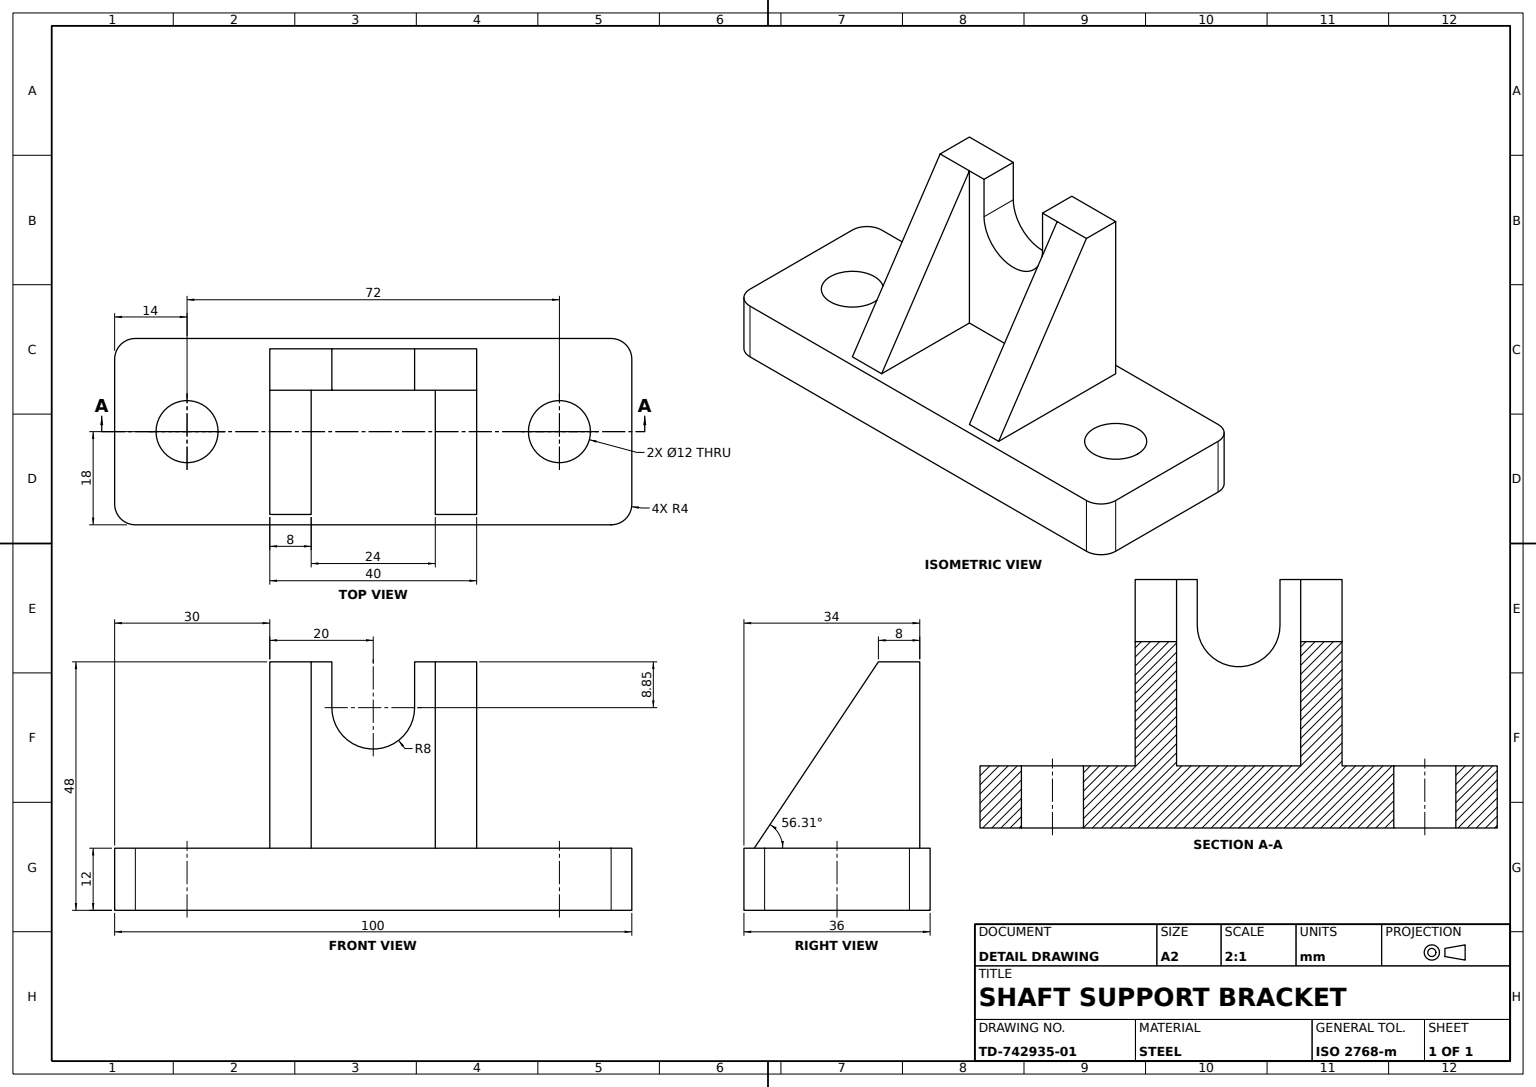
SolidWorks part; units mm, degrees
material "Plain Carbon Steel"
ref_plane "Front Plane" through (0, 0, 0) normal (0, 0, 1) x (1, 0, 0)
ref_plane "Top Plane" through (0, 0, 0) normal (0, 1, 0) x (1, 0, 0)
ref_plane "Right Plane" through (0, 0, 0) normal (1, 0, 0) x (0, 0, -1)
sketch "Base Plate Profile" plane through (0, 0, 0) normal (0, 0, 1) x (1, 0, 0)
  line L0 (0, 0) -> (50, 0)
  line L1 (50, 0) -> (50, 12)
  line L2 (50, 12) -> (-50, 12)
  line L3 (-50, 12) -> (-50, 0)
  line L4 (-50, 0) -> (0, 0)
  dimension "D1" = 100
  dimension "D2" = 12
  dimension "D3" = 50
extrude "Base Plate" add sketch "Base Plate Profile" along normal mid plane 36
sketch "Base Corners and Holes Sketch" plane through (0, 12, 0) normal (0, 1, 0) x (1, 0, 0)
  line L2 (-50, -14) -> (-50, -18)
  line L4 (-50, -18) -> (-46, -18)
  line L5 (50, 18) -> (-50, 18) construction
  line L6 (0, 18) -> (0, 0) construction
  line L7 (0, 0) -> (-26.4837, 0) construction
  line L8 (50, -14) -> (50, -18)
  line L9 (50, -18) -> (46, -18)
  line L10 (50, 14) -> (50, 18)
  line L11 (50, 18) -> (46, 18)
  line L12 (-50, 18) -> (-46, 18)
  line L13 (-50, 14) -> (-50, 18)
  arc A0 (-50, -14) -> (-46, -18) centre (-46, -14) ccw
  arc A1 (50, -14) -> (46, -18) centre (46, -14) cw
  arc A2 (50, 14) -> (46, 18) centre (46, 14) ccw
  arc A3 (-50, 14) -> (-46, 18) centre (-46, 14) cw
  point P10 (-50, -18)
  dimension "D1" = 4
  dimension "D2" = 48.0833
extrude "Base Corners and Mounting Holes" cut sketch "Base Corners and Holes Sketch" against normal blind 36
sketch "Base Relief Sketch" plane through (0, 12, 0) normal (0, 1, 0) x (1, 0, 0)
  line L0 (-50, -14) -> (-36, -14) construction
  line L1 (-36, -14) -> (-36, 0) construction
  line L2 (0, 0) -> (0, 18) construction
  line L3 (46, 18) -> (-46, 18) construction
  circle A0 centre (-36, 0) radius 6
  circle A1 centre (36, 0) radius 6
  dimension "D1" = 12
  dimension "D2" = 14
  dimension "D3" = 36
extrude "Base Relief Cut" cut sketch "Base Relief Sketch" against normal blind 36
sketch "Upright Profile" plane through (0, 0, 18) normal (0, 0, 1) x (1, 0, 0)
  line L0 (0, 0) -> (0, 36) construction
  line L1 (8, 39.151) -> (8, 48)
  line L3 (-8, 39.151) -> (-8, 48)
  line L4 (-20, 48) -> (-20, 12)
  line L5 (-8, 48) -> (-20, 48)
  line L6 (46, 12) -> (-46, 12) construction
  line L7 (-20, 12) -> (20, 12)
  line L10 (8, 48) -> (20, 48)
  line L12 (20, 48) -> (20, 12)
  arc A0 (8, 39.151) -> (-8, 39.151) centre (0, 39.151) cw
  dimension "D1" = 8
  dimension "D2" = 12
  dimension "D3" = 36
  dimension "D4" = 8.849
  dimension "D5" = 12
  dimension "D6" = 40
  dimension "D7" = 36
  dimension "D8" = 20
extrude "Support Upright" add sketch "Upright Profile" against normal blind 34
sketch "Upright Taper Sketch" plane through (-20, 0, 0) normal (-1, 0, 0) x (0, 0, 1)
  line L0 (-8, 48) -> (18, 48)
  line L1 (-16, 48) -> (18, 48) construction
  line L2 (-8, 48) -> (16, 12)
  line L3 (-16, 12) -> (18, 12) construction
  line L7 (18, 48) -> (18, 12)
  line L8 (18, 12) -> (16, 12)
  dimension "D1" = 43.2666
  dimension "D2" = 48.6621
extrude "Upright Taper Cut" cut sketch "Upright Taper Sketch" against normal through all
sketch "Bearing Seat Sketch" plane through (0, 0, 0) normal (1, 0, 0) x (0, 0, -1)
  line L0 (8, 48) -> (8, 12)
  line L1 (16, 12) -> (-16, 12) construction
  line L2 (8, 12) -> (-16, 12)
  line L3 (-16, 12) -> (8, 48)
extrude "Bearing Seat Cut" cut sketch "Bearing Seat Sketch" against normal mid plane 24
